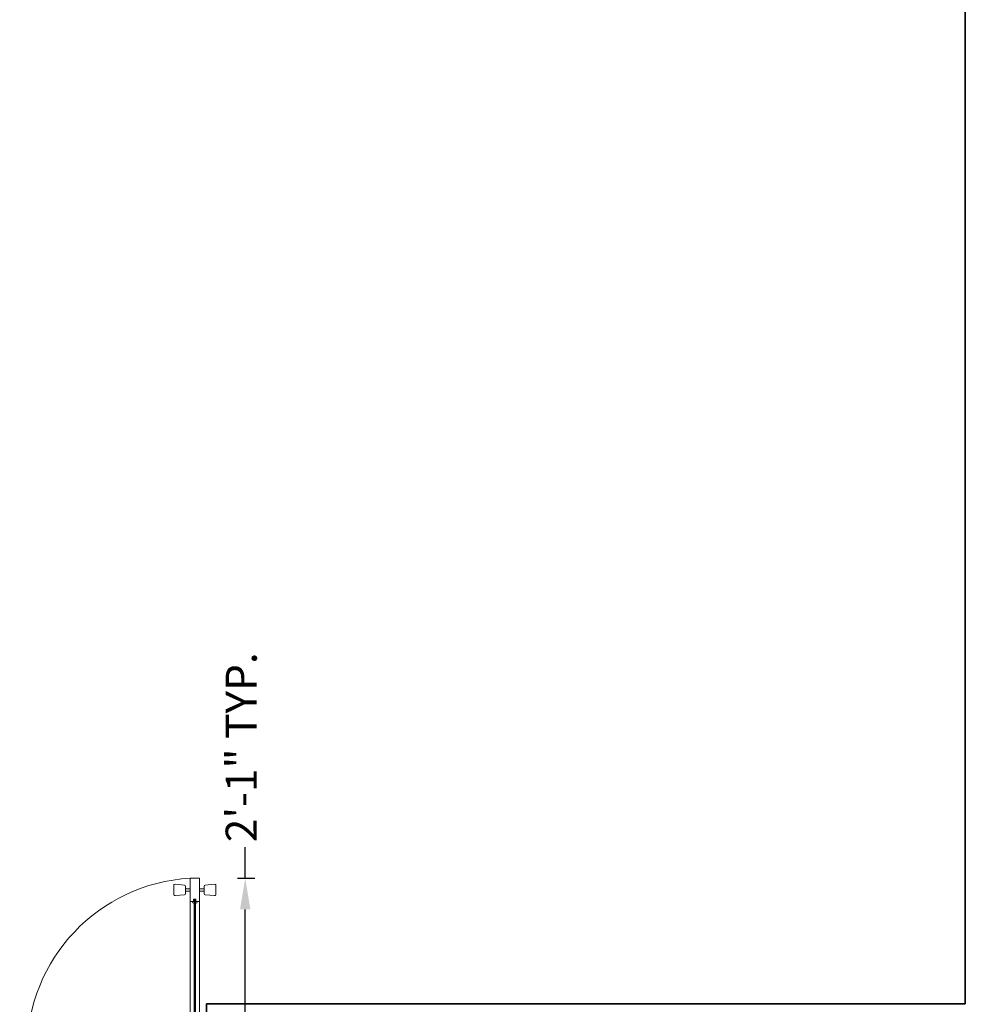
# Model space of a CAD drawing. Units: inches. Extents: x -638 to 186, y -762 to 59.
# Tile 4 of 31: x -287 to -164, y -539 to -413. Entities that reach past the tile are written whole.
import ezdxf

# ---------------------------------------------------------------- set-up
doc = ezdxf.new("R2010")
doc.units = ezdxf.units.IN
for name, color, linetype, lineweight in [('A-ANNO-DIMS', 2, 'Continuous', 18), ('A-DOOR', 3, 'Continuous', 18), ('wall', 7, 'Continuous', 35)]:
    doc.layers.add(name, color=color, linetype=linetype, lineweight=lineweight)
doc.styles.get("Standard").update_dxf_attribs({"font": 'arial.ttf'})
doc.dimstyles.new('ISO-25', dxfattribs={"dimtxt": 4, "dimasz": 4, "dimexe": 1.25, "dimexo": 0.625, "dimtad": 0, "dimlunit": 4, "dimtxsty": 'Standard', "dimcen": 2.5, "dimclrt": 256, "dimadec": 0, "dimazin": 0, "dimtfac": 1, "dimtmove": 0, "dimatfit": 3, "dimfxl": 1, "dimfxlon": 1, "dimarcsym": 0})

# ---------------------------------------------------------------- blocks, each defined once
blk = doc.blocks.new('DOOR-ENTRY-24IN-LEAF')
for p, q in [((21.85, 22.14), (21.85, 5.99)), ((22.38, 22.44), (22.37, 5.69)), ((22.45, 22.44), (22.45, 5.69)), ((22.53, 22.44), (22.52, 5.69)), ((23.05, 22.14), (23.04, 5.99)), ((1.5, 1.8), (22.44, 1.8))]:
    blk.add_line(p, q)
for points in [[(21.11, 23.03), (19.91, 22.91, -0.443716), (19.75, 23.06), (19.75, 24.22, -0.443716), (19.91, 24.37), (21.11, 24.25, -0.385314), (21.24, 24.1), (21.24, 23.18, -0.385314)], [(23.79, 23.03), (24.99, 22.91, 0.443716), (25.15, 23.06), (25.16, 24.22, 0.443716), (24.99, 24.37), (23.79, 24.25, 0.385314), (23.66, 24.1), (23.66, 23.18, 0.385314)]]:
    blk.add_lwpolyline(points, format="xyb", close=True)
for points in [[(22.3, 22.14), (21.85, 22.14), (21.85, 25.14), (23.05, 25.14), (23.05, 22.14), (22.6, 22.14), (22.6, 22.44), (22.3, 22.44), (22.3, 22.14)], [(22.3, 5.99), (21.85, 5.99), (21.85, 2.99), (23.04, 2.99), (23.04, 5.99), (22.59, 5.99), (22.59, 5.69), (22.3, 5.69), (22.3, 5.99)], [(0.9, 3), (0.9, 1.8), (1.5, 1.8), (1.5, 0.01), (0, 0.01), (0, 3), (0.9, 3)], [(23.04, 2.99), (23.04, 1.8), (22.44, 1.8), (22.44, 0), (23.94, 0), (23.94, 2.99), (23.04, 2.99)]]:
    blk.add_lwpolyline(points)
for points in [[(21.85, 23.49), (21.24, 23.49), (21.24, 23.79), (21.85, 23.79)], [(23.05, 23.49), (23.66, 23.49), (23.66, 23.79), (23.05, 23.79)]]:
    blk.add_lwpolyline(points, close=True)
for centre, radius, start, end in [((23.1, 2.97), 22.21, 93.2293, 179.917), ((22.36, 22.17), 0.247, 186.4162, 273.2718), ((22.54, 22.17), 0.247, 266.6922, 353.5478), ((22.36, 5.96), 0.247, 86.6922, 173.5478), ((22.53, 5.96), 0.247, 6.4162, 93.2718)]:
    blk.add_arc(centre, radius, start, end)
blk = doc.blocks.new('*D30')
at = {"layer": 'A-ANNO-DIMS', "color": 0, "lineweight": -2, "transparency": 16777216}
for p, q in [((-257.54, -522.91), (-257.54, -518.91)), ((-258.54, -522.91), (-256.29, -522.91)), ((-257.54, -544.05), (-257.54, -526.91)), ((-258.54, -548.05), (-256.29, -548.05))]:
    blk.add_line(p, q, dxfattribs=at)
at = {"layer": 'A-ANNO-DIMS', "color": 0, "lineweight": 30, "transparency": 16777216}
for points in [[(-258.21, -526.91), (-256.88, -526.91), (-257.54, -522.91)], [(-258.21, -544.05), (-256.88, -544.05), (-257.54, -548.05)]]:
    blk.add_solid(points, dxfattribs=at)
at = {"layer": 'Defpoints', "color": 0, "lineweight": 30, "transparency": 16777216}
for p in [(-261.32, -522.91), (-257.54, -522.91), (-261.32, -548.05)]:
    blk.add_point(p, dxfattribs=at)
at = {"layer": 'A-ANNO-DIMS', "transparency": 16777216, "insert": (-257.54, -506.06), "char_height": 4, "attachment_point": 5, "rotation": 90}
blk.add_mtext('2\'-1" TYP.', dxfattribs=at)
blk = doc.blocks.new('*D38')
at = {"layer": 'A-ANNO-DIMS', "color": 0, "lineweight": -2, "transparency": 16777216}
for p, q in [((182.66, -280.53), (184.91, -280.53)), ((183.66, -284.53), (183.66, -371.73)), ((183.66, -473.53), (183.66, -386.34)), ((182.66, -477.53), (184.91, -477.53))]:
    blk.add_line(p, q, dxfattribs=at)
at = {"layer": 'A-ANNO-DIMS', "color": 0, "lineweight": 30, "transparency": 16777216}
for points in [[(183, -284.53), (184.33, -284.53), (183.66, -280.53)], [(183, -473.53), (184.33, -473.53), (183.66, -477.53)]]:
    blk.add_solid(points, dxfattribs=at)
at = {"layer": 'Defpoints', "color": 0, "lineweight": 30, "transparency": 16777216}
for p in [(-404.53, -280.53), (-404.53, -477.53), (183.66, -477.53)]:
    blk.add_point(p, dxfattribs=at)
at = {"layer": 'A-ANNO-DIMS', "transparency": 16777216, "insert": (183.66, -379.03), "char_height": 4, "attachment_point": 5, "rotation": 90}
blk.add_mtext('16\'-5"', dxfattribs=at)
blk = doc.blocks.new('*D39')
at = {"layer": 'A-ANNO-DIMS', "color": 0, "lineweight": -2, "transparency": 16777216}
for p, q in [((-344.53, -751.58), (-344.53, -753.83)), ((-271.53, -751.58), (-271.53, -753.83)), ((-340.53, -752.58), (-313.98, -752.58)), ((-275.53, -752.58), (-302.07, -752.58))]:
    blk.add_line(p, q, dxfattribs=at)
at = {"layer": 'A-ANNO-DIMS', "color": 0, "lineweight": 30, "transparency": 16777216}
for points in [[(-340.53, -751.92), (-340.53, -753.25), (-344.53, -752.58)], [(-275.53, -751.92), (-275.53, -753.25), (-271.53, -752.58)]]:
    blk.add_solid(points, dxfattribs=at)
at = {"layer": 'Defpoints', "color": 0, "lineweight": 30, "transparency": 16777216}
for p in [(-344.53, -214.53), (-271.53, -214.53), (-271.53, -752.58)]:
    blk.add_point(p, dxfattribs=at)
at = {"layer": 'A-ANNO-DIMS', "transparency": 16777216, "insert": (-308.03, -752.58), "char_height": 4, "attachment_point": 5}
blk.add_mtext('6\'-1"', dxfattribs=at)

msp = doc.modelspace()

# ---------------------------------------------------------------- linework, layer by layer
at = {"layer": 'wall'}
for p, q in [((-165.026, -408.033), (-165.026, -539.033)), ((-165.026, -539.033), (-262.526, -539.033)), ((-262.526, -539.033), (-262.526, -548.033))]:
    msp.add_line(p, q, dxfattribs=at)

# ---------------------------------------------------------------- block references
at = {"layer": 'A-DOOR'}
msp.add_blockref('DOOR-ENTRY-24IN-LEAF', (-286.471, -548.048), dxfattribs=at)

# ---------------------------------------------------------------- dimensions: what is measured, and where the dimension line sits
at = {"layer": 'A-ANNO-DIMS'}
dim = msp.add_linear_dim(base=(-271.526, -752.583), p1=(-344.526, -214.533), p2=(-271.526, -214.533), dimstyle='ISO-25', override={"dimdec": 1, "dimlfac": 1, "dimrnd": 0, "dimzin": 1, "dimdsep": 46, "dimlunit": 4, "dimfrac": 2}, dxfattribs=at)
dim.commit()
dim.dimension.update_dxf_attribs({"geometry": '*D39', "text_midpoint": (-308.026, -752.583)})
dim = msp.add_linear_dim(base=(183.663, -477.533), p1=(-404.526, -280.533), p2=(-404.526, -477.533), angle=90, dimstyle='ISO-25', override={"dimdec": 1, "dimlfac": 1, "dimrnd": 0, "dimzin": 1, "dimdsep": 46, "dimlunit": 4, "dimfrac": 2}, dxfattribs=at)
dim.commit()
dim.dimension.update_dxf_attribs({"geometry": '*D38', "text_midpoint": (183.663, -379.033)})
dim = msp.add_linear_dim(base=(-257.543, -522.911), p1=(-261.316, -548.048), p2=(-261.316, -522.911), angle=90, text='<> TYP.', dimstyle='ISO-25', override={"dimdec": 1, "dimlfac": 1, "dimrnd": 0, "dimzin": 1, "dimdsep": 46, "dimlunit": 4, "dimfrac": 2}, dxfattribs=at)
dim.commit()
dim.dimension.update_dxf_attribs({"geometry": '*D30', "text_midpoint": (-257.543, -506.061)})

doc.saveas('drawing.dxf')
